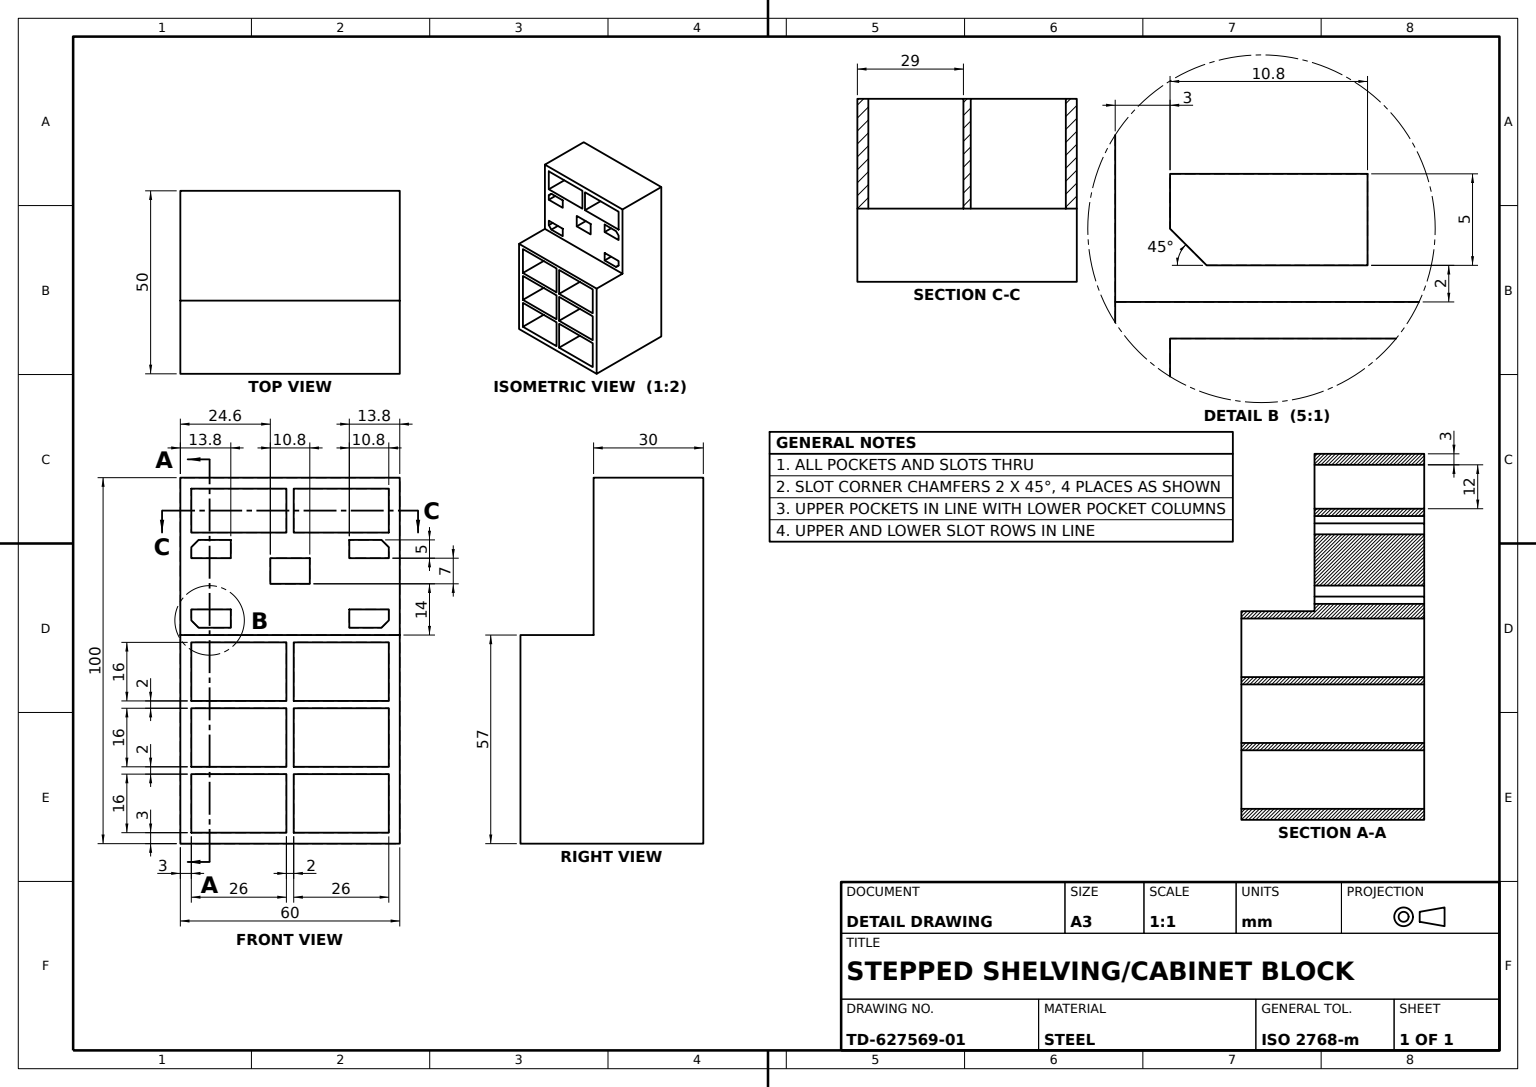
SolidWorks part; units mm, degrees
material "Plain Carbon Steel"
ref_plane "Front Plane" through (0, 0, 0) normal (0, 0, 1) x (1, 0, 0)
ref_plane "Top Plane" through (0, 0, 0) normal (0, 1, 0) x (1, 0, 0)
ref_plane "Right Plane" through (0, 0, 0) normal (1, 0, 0) x (0, 0, -1)
sketch "Base Block Sketch" plane through (0, 0, 0) normal (0, 0, 1) x (1, 0, 0)
  line L1 (-30, -50) -> (30, -50)
  line L2 (-30, -50) -> (-30, 50)
  line L3 (-30, 50) -> (30, 50)
  line L4 (30, -50) -> (30, 50)
  line L5 (-30, -50) -> (30, 50) construction
  line L6 (-30, 50) -> (30, -50) construction
  point P0 (0, 0)
  dimension "D1" = 60
  dimension "D2" = 100
extrude "Base Block" add sketch "Base Block Sketch" along normal blind 30
sketch "Lower Cell Pockets Sketch" plane through (0, 0, 30) normal (0, 0, 1) x (1, 0, 0)
  line L0 (-27, 47) -> (-27, 35)
  line L3 (27, 47) -> (1, 47)
  line L12 (30, -50) -> (30, 50) construction
  line L13 (30, 50) -> (-30, 50) construction
  line L15 (0, 15.2663) -> (0, 61.1845) construction
  line L16 (-21.7881, 47) -> (-1, 47)
  line L18 (-27, 35) -> (-1, 35)
  line L19 (-1, 47) -> (-1, 35)
  line L20 (1, 47) -> (26.1586, 47)
  line L21 (1, 47) -> (1, 35)
  line L22 (1, 35) -> (27, 35)
  line L24 (-41.0812, 35) -> (40.5895, 35) construction
  line L25 (-1, 47) -> (-27, 47)
  line L32 (27, 35) -> (27, 47)
  point P4 (-27, -47)
  point P6 (27, -47)
  dimension "D3" = 51.7881
  dimension "D4" = 3
  dimension "D5" = 2
  dimension "D6" = 12
  dimension "D1" = 3
  dimension "D2" = 3.8414
extrude "Lower Cell Pockets" cut sketch "Lower Cell Pockets Sketch" against normal through all contours L22 L32 L3 L21 | L16 L25 L0 L18 L19
sketch "Upper Step Sketch" plane through (0, 0, 30) normal (0, 0, 1) x (1, 0, 0)
  line L0 (30, -50) -> (30, 50) construction
  line L1 (-30, -50) -> (30, -50)
  line L2 (-30, -50) -> (-30, 7)
  line L3 (-30, 7) -> (30, 7)
  line L4 (30, -50) -> (30, 7)
  dimension "D1" = 57
extrude "Upper Step Boss" add sketch "Upper Step Sketch" along normal blind 20
sketch "Upper Cell Pockets Sketch" plane through (0, 0, 50) normal (0, 0, 1) x (1, 0, 0)
  line L0 (0, 18.7903) -> (0, -56.0915) construction
  line L1 (-27, 35) -> (-27, -47) construction
  line L2 (-27, 35) -> (-1, 35) construction
  line L3 (-30, -50) -> (30, -50) construction
  line L4 (-27, -47) -> (26.8233, -47) construction
  line L5 (26.8233, -47) -> (27, 35) construction
  line L6 (30, 7) -> (-30, 7) construction
  line L7 (-27, 5) -> (-1, 5)
  line L8 (-27, 5) -> (-27, -11)
  line L9 (-27, -11) -> (-1, -11)
  line L10 (-1, 5) -> (-1, -11)
  line L11 (1, -11) -> (27, -11)
  line L12 (1, 5) -> (27, 5)
  line L13 (27, 5) -> (27, -11)
  line L14 (1, 5) -> (1, -11)
  line L15 (1, -29) -> (27, -29)
  line L16 (1, -13) -> (27, -13)
  line L17 (27, -13) -> (27, -29)
  line L18 (1, -13) -> (1, -29)
  line L19 (1, -47) -> (27, -47)
  line L20 (1, -31) -> (27, -31)
  line L21 (27, -31) -> (27, -47)
  line L22 (1, -31) -> (1, -47)
  line L23 (-27, -29) -> (-1, -29)
  line L24 (-27, -13) -> (-1, -13)
  line L25 (-1, -13) -> (-1, -29)
  line L26 (-27, -13) -> (-27, -29)
  line L27 (-27, -47) -> (-1, -47)
  line L28 (-27, -31) -> (-1, -31)
  line L29 (-1, -31) -> (-1, -47)
  line L30 (-27, -31) -> (-27, -47)
  dimension "D1" = 3
  dimension "D2" = 2
  dimension "D3" = 16
  dimension "D4" = 1
  dimension "D7" = 26
  dimension "D8" = 53.8233
  dimension "D9" = 2
  dimension "D5" = 2
  dimension "D6" = 3
extrude "Upper Cell Pockets" cut sketch "Upper Cell Pockets Sketch" against normal through all
sketch "Back Wall Slots Sketch" plane through (0, 0, 30) normal (0, 0, 1) x (1, 0, 0)
  line L0 (-27, 35) -> (-27, 5) construction
  line L1 (-1, 5) -> (-27, 5) construction
  line L2 (27, 35) -> (27, 3.7612) construction
  line L3 (27, -11) -> (27, 5) construction
  line L4 (-27, 35) -> (-1, 35) construction
  line L5 (-27, 33) -> (27, 33)
  line L6 (-27, 33) -> (-27, 9)
  line L7 (-27, 9) -> (27, 9)
  line L8 (27, 33) -> (27, 9)
  line L9 (30, 7) -> (-30, 7) construction
  line L10 (-25, 9) -> (-27, 11)
  line L11 (0, 0) -> (0, 39.8004) construction
  line L12 (25, 9) -> (27, 11)
  line L13 (-27, 21) -> (27, 21) construction
  line L14 (25, 33) -> (27, 31)
  line L15 (-25, 33) -> (-27, 31)
  line L16 (-27, 28) -> (27, 28)
  line L17 (-27, 21) -> (27, 21)
  line L18 (-27, 14) -> (27, 14)
  line L19 (-16.2, 33) -> (-16.2, 9)
  line L20 (-5.4, 33) -> (-5.4, 9)
  line L21 (5.4, 33) -> (5.4, 9)
  line L22 (16.2, 33) -> (16.2, 9)
  dimension "D1" = 2
  dimension "D2" = 2
  dimension "D3" = 45
  dimension "D4" = 2
  dimension "D5" = 10.8
  dimension "D6" = 10.8
  dimension "D7" = 10.8
  dimension "D8" = 10.8
  dimension "D9" = 5
  dimension "D10" = 5
extrude "Back Wall Slots" cut sketch "Back Wall Slots Sketch" against normal through all contours L18 L22 L7 L12 L8 | L21 L16 L20 L17 | L19 L5 L15 L6 L16 | L5 L22 L16 L8 L14 | L19 L18 L6 L10 L7
